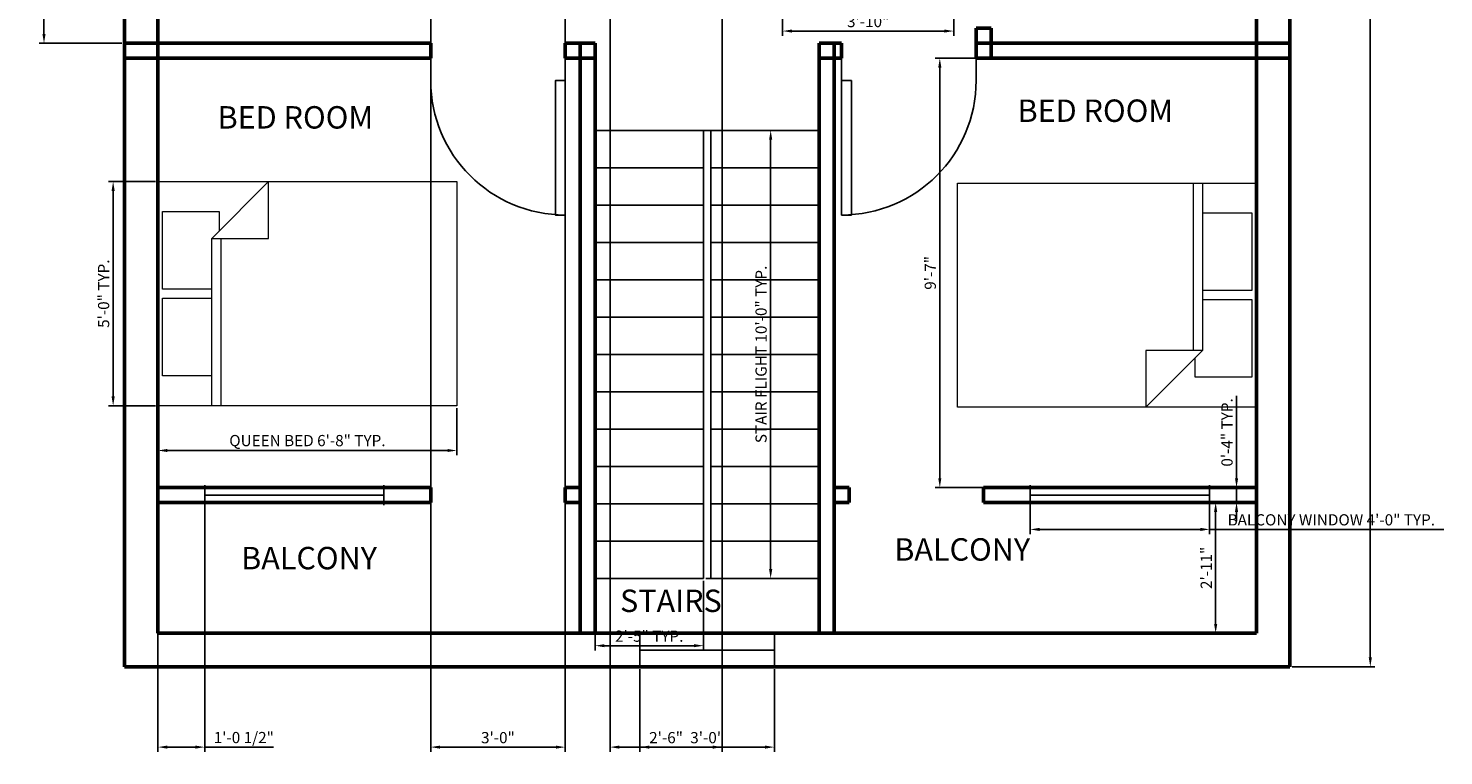
# Model space of a CAD drawing. Units: inches. Extents: x 1767 to 2185, y 3382 to 3854.
# Tile 1 of 4: x 1806 to 2185, y 3382 to 3577. Entities that reach past the tile are written whole.
import ezdxf

# ---------------------------------------------------------------- set-up
doc = ezdxf.new("R2010")
doc.units = ezdxf.units.IN
for name, color, linetype, lineweight in [('A-ANNO-DIMS', 2, 'Continuous', 18), ('A-AREA-IDEN', 7, 'Continuous', 25), ('A-DOOR', 3, 'Continuous', 25), ('A-FLOR-STRS', 7, 'Continuous', 25), ('A-FURN', 8, 'Continuous', 18), ('A-GLAZ', 4, 'Continuous', 25), ('A-WALL', 7, 'Continuous', 50)]:
    doc.layers.add(name, color=color, linetype=linetype, lineweight=lineweight)
doc.styles.get("Standard").update_dxf_attribs({"font": 'arial.ttf'})
doc.dimstyles.new('ISO-25', dxfattribs={"dimtxt": 3, "dimasz": 2.5, "dimexe": 1.25, "dimexo": 0.625, "dimtad": 1, "dimdec": 0, "dimlunit": 3, "dimtxsty": 'Standard', "dimcen": 2.5, "dimadec": 0, "dimazin": 0, "dimtfac": 1, "dimtdec": 0, "dimtmove": 0, "dimatfit": 3, "dimfxl": 1, "dimarcsym": 0})

# ---------------------------------------------------------------- blocks, each defined once
blk = doc.blocks.new('*U2')
for p, q in [((0, 0), (0, -100)), ((600, 0), (600, -100))]:
    blk.add_line(p, q)
blk.add_lwpolyline([(0, 0), (0, 600), (43.75, 600), (43.75, 0)], close=True)
blk.add_arc((0, 0), 600, 0, 90)
blk = doc.blocks.new('*U4')
for p, q in [((0, 100), (0, 0)), ((900, 100), (900, 0)), ((0, 50), (900, 50))]:
    blk.add_line(p, q)
blk = doc.blocks.new('Bed - Queen')
for p, q in [((0, -80.00003), (0, 0)), ((0, 0), (59.99999, 0)), ((59.99999, 0), (59.99999, -80.00003)), ((7.99999, -1.2), (28.79998, -1.2)), ((7.99999, -14.4), (7.99999, -1.2)), ((28.79998, -1.2), (28.79998, -14.4)), ((31.19999, -1.2), (51.99999, -1.2)), ((31.19999, -14.4), (31.19999, -1.2)), ((51.99999, -1.2), (51.99999, -16.4)), ((0, -14.4), (44.8, -14.4)), ((59.99999, -29.6), (44.8, -14.4)), ((44.8, -14.4), (44.8, -29.6)), ((44.8, -16.8), (0, -16.8)), ((51.99999, -16.4), (46.79936, -16.4)), ((44.8, -29.6), (59.99999, -29.6)), ((59.99999, -80.00003), (0, -80.00003))]:
    blk.add_line(p, q)
blk = doc.blocks.new('*D18')
at = {"layer": 'A-ANNO-DIMS', "color": 0, "lineweight": -2, "transparency": 16777216}
for p, q in [((2134.53, 3569.15), (2049.19, 3569.15)), ((2050.44, 3566.65), (2050.44, 3456.65)), ((2134.53, 3454.15), (2049.19, 3454.15))]:
    blk.add_line(p, q, dxfattribs=at)
at = {"layer": 'A-ANNO-DIMS', "color": 0, "transparency": 16777216}
for points in [[(2050.02, 3566.65), (2050.85, 3566.65), (2050.44, 3569.15)], [(2050.02, 3456.65), (2050.85, 3456.65), (2050.44, 3454.15)]]:
    blk.add_solid(points, dxfattribs=at)
at = {"layer": 'Defpoints', "color": 0, "transparency": 16777216}
for p in [(2135.16, 3569.15), (2050.44, 3454.15), (2135.16, 3454.15)]:
    blk.add_point(p, dxfattribs=at)
at = {"layer": 'A-ANNO-DIMS', "color": 0, "transparency": 16777216, "insert": (2048.28, 3511.65), "char_height": 3, "attachment_point": 5, "rotation": 90}
blk.add_mtext('9\'-7"', dxfattribs=at)
blk = doc.blocks.new('*D19')
at = {"layer": 'A-ANNO-DIMS', "color": 0, "lineweight": -2, "transparency": 16777216}
for p, q in [((2134.53, 3450.15), (2123.02, 3450.15)), ((2124.27, 3417.65), (2124.27, 3447.65)), ((2134.53, 3415.15), (2123.02, 3415.15))]:
    blk.add_line(p, q, dxfattribs=at)
at = {"layer": 'A-ANNO-DIMS', "color": 0, "transparency": 16777216}
for points in [[(2123.85, 3447.65), (2124.69, 3447.65), (2124.27, 3450.15)], [(2123.85, 3417.65), (2124.69, 3417.65), (2124.27, 3415.15)]]:
    blk.add_solid(points, dxfattribs=at)
at = {"layer": 'Defpoints', "color": 0, "transparency": 16777216}
for p in [(2124.27, 3450.15), (2135.16, 3450.15), (2135.16, 3415.15)]:
    blk.add_point(p, dxfattribs=at)
at = {"layer": 'A-ANNO-DIMS', "color": 0, "transparency": 16777216, "insert": (2122.14, 3432.65), "char_height": 3, "attachment_point": 5, "rotation": 90}
blk.add_mtext('2\'-11"', dxfattribs=at)
blk = doc.blocks.new('STAIR-FLIGHT-29IN-13-TREAD')
for p, q in [((0, 120), (29, 120)), ((29, 0), (29, 120)), ((0, 110), (29, 110)), ((0, 100), (29, 100)), ((0, 90), (29, 90)), ((0, 80), (29, 80)), ((0, 70), (29, 70)), ((0, 60), (29, 60)), ((0, 50), (29, 50)), ((0, 40), (29, 40)), ((0, 30), (29, 30)), ((0, 20), (29, 20)), ((0, 10), (29, 10)), ((0, 0), (29, 0))]:
    blk.add_line(p, q)
blk = doc.blocks.new('WIN-OPENING-48IN-WALL-4IN')
for p, q in [((48, 4), (0, 4)), ((0, 4), (0, 0)), ((48, 0), (48, 4))]:
    blk.add_line(p, q)
blk = doc.blocks.new('*D23')
at = {"layer": 'A-ANNO-DIMS', "color": 0, "lineweight": -2, "transparency": 16777216}
for p, q in [((1841.16, 3475.46), (1841.16, 3462.83)), ((1921.16, 3475.46), (1921.16, 3462.83)), ((1918.66, 3464.08), (1843.66, 3464.08))]:
    blk.add_line(p, q, dxfattribs=at)
at = {"layer": 'A-ANNO-DIMS', "color": 0, "transparency": 16777216}
for points in [[(1843.66, 3464.5), (1843.66, 3463.67), (1841.16, 3464.08)], [(1918.66, 3464.5), (1918.66, 3463.67), (1921.16, 3464.08)]]:
    blk.add_solid(points, dxfattribs=at)
at = {"layer": 'Defpoints', "color": 0, "transparency": 16777216}
for p in [(1841.16, 3476.08), (1921.16, 3476.08), (1841.16, 3464.08)]:
    blk.add_point(p, dxfattribs=at)
at = {"layer": 'A-ANNO-DIMS', "color": 0, "transparency": 16777216, "insert": (1881.16, 3466.35), "char_height": 3, "attachment_point": 5}
blk.add_mtext('QUEEN BED 6\'-8" TYP.', dxfattribs=at)
blk = doc.blocks.new('*D24')
at = {"layer": 'A-ANNO-DIMS', "color": 0, "lineweight": -2, "transparency": 16777216}
for p, q in [((1840.53, 3536.08), (1827.91, 3536.08)), ((1829.16, 3478.58), (1829.16, 3533.58)), ((1840.53, 3476.08), (1827.91, 3476.08))]:
    blk.add_line(p, q, dxfattribs=at)
at = {"layer": 'A-ANNO-DIMS', "color": 0, "transparency": 16777216}
for points in [[(1828.74, 3533.58), (1829.58, 3533.58), (1829.16, 3536.08)], [(1828.74, 3478.58), (1829.58, 3478.58), (1829.16, 3476.08)]]:
    blk.add_solid(points, dxfattribs=at)
at = {"layer": 'Defpoints', "color": 0, "transparency": 16777216}
for p in [(1829.16, 3536.08), (1841.16, 3536.08), (1841.16, 3476.08)]:
    blk.add_point(p, dxfattribs=at)
at = {"layer": 'A-ANNO-DIMS', "color": 0, "transparency": 16777216, "insert": (1827, 3506.08), "char_height": 3, "attachment_point": 5, "rotation": 90}
blk.add_mtext('5\'-0" TYP.', dxfattribs=at)
blk = doc.blocks.new('*D25')
at = {"layer": 'A-ANNO-DIMS', "color": 0, "lineweight": -2, "transparency": 16777216}
for p, q in [((1987.78, 3549.81), (2006.41, 3549.81)), ((2005.16, 3432.31), (2005.16, 3547.31)), ((1987.78, 3429.81), (2006.41, 3429.81))]:
    blk.add_line(p, q, dxfattribs=at)
at = {"layer": 'A-ANNO-DIMS', "color": 0, "transparency": 16777216}
for points in [[(2004.74, 3547.31), (2005.58, 3547.31), (2005.16, 3549.81)], [(2004.74, 3432.31), (2005.58, 3432.31), (2005.16, 3429.81)]]:
    blk.add_solid(points, dxfattribs=at)
at = {"layer": 'Defpoints', "color": 0, "transparency": 16777216}
for p in [(1987.16, 3549.81), (2005.16, 3549.81), (1987.16, 3429.81)]:
    blk.add_point(p, dxfattribs=at)
at = {"layer": 'A-ANNO-DIMS', "color": 0, "transparency": 16777216, "insert": (2002.98, 3489.81), "char_height": 3, "attachment_point": 5, "rotation": 90}
blk.add_mtext('STAIR FLIGHT 10\'-0" TYP.', dxfattribs=at)
blk = doc.blocks.new('*D26')
at = {"layer": 'A-ANNO-DIMS', "color": 0, "lineweight": -2, "transparency": 16777216}
for p, q in [((1958.16, 3429.19), (1958.16, 3410.56)), ((1987.16, 3429.19), (1987.16, 3410.56)), ((1960.66, 3411.81), (1984.66, 3411.81))]:
    blk.add_line(p, q, dxfattribs=at)
at = {"layer": 'A-ANNO-DIMS', "color": 0, "transparency": 16777216}
for points in [[(1960.66, 3412.23), (1960.66, 3411.4), (1958.16, 3411.81)], [(1984.66, 3412.23), (1984.66, 3411.4), (1987.16, 3411.81)]]:
    blk.add_solid(points, dxfattribs=at)
at = {"layer": 'Defpoints', "color": 0, "transparency": 16777216}
for p in [(1958.16, 3429.81), (1987.16, 3429.81), (1987.16, 3411.81)]:
    blk.add_point(p, dxfattribs=at)
at = {"layer": 'A-ANNO-DIMS', "color": 0, "transparency": 16777216, "insert": (1972.66, 3413.97), "char_height": 3, "attachment_point": 5}
blk.add_mtext('2\'-5" TYP.', dxfattribs=at)
blk = doc.blocks.new('*D29')
at = {"layer": 'A-ANNO-DIMS', "color": 0, "lineweight": -2, "transparency": 16777216}
for p, q in [((2074.66, 3449.53), (2074.66, 3441.7)), ((2122.66, 3449.53), (2122.66, 3441.7)), ((2077.16, 3442.95), (2120.16, 3442.95)), ((2122.66, 3442.95), (2185.31, 3442.95))]:
    blk.add_line(p, q, dxfattribs=at)
at = {"layer": 'A-ANNO-DIMS', "color": 0, "transparency": 16777216}
for points in [[(2077.16, 3443.37), (2077.16, 3442.53), (2074.66, 3442.95)], [(2120.16, 3443.37), (2120.16, 3442.53), (2122.66, 3442.95)]]:
    blk.add_solid(points, dxfattribs=at)
at = {"layer": 'Defpoints', "color": 0, "transparency": 16777216}
for p in [(2074.66, 3450.15), (2122.66, 3450.15), (2122.66, 3442.95)]:
    blk.add_point(p, dxfattribs=at)
at = {"layer": 'A-ANNO-DIMS', "color": 0, "transparency": 16777216, "insert": (2155.23, 3445.13), "char_height": 3, "attachment_point": 5}
blk.add_mtext('BALCONY WINDOW 4\'-0" TYP.', dxfattribs=at)
blk = doc.blocks.new('*D30')
at = {"layer": 'A-ANNO-DIMS', "color": 0, "lineweight": -2, "transparency": 16777216}
for p, q in [((2129.86, 3456.65), (2129.86, 3478.69)), ((2123.28, 3454.15), (2131.11, 3454.15)), ((2129.86, 3450.15), (2129.86, 3454.15)), ((2123.28, 3450.15), (2131.11, 3450.15)), ((2129.86, 3447.65), (2129.86, 3445.15))]:
    blk.add_line(p, q, dxfattribs=at)
at = {"layer": 'A-ANNO-DIMS', "color": 0, "transparency": 16777216}
for points in [[(2129.44, 3456.65), (2130.28, 3456.65), (2129.86, 3454.15)], [(2129.44, 3447.65), (2130.28, 3447.65), (2129.86, 3450.15)]]:
    blk.add_solid(points, dxfattribs=at)
at = {"layer": 'Defpoints', "color": 0, "transparency": 16777216}
for p in [(2122.66, 3454.15), (2129.86, 3454.15), (2122.66, 3450.15)]:
    blk.add_point(p, dxfattribs=at)
at = {"layer": 'A-ANNO-DIMS', "color": 0, "transparency": 16777216, "insert": (2127.7, 3468.92), "char_height": 3, "attachment_point": 5, "rotation": 90}
blk.add_mtext('0\'-4" TYP.', dxfattribs=at)
blk = doc.blocks.new('*D32')
at = {"layer": 'A-ANNO-DIMS', "color": 0, "lineweight": -2, "transparency": 16777216}
for p, q in [((2008.34, 3587.16), (2008.34, 3575.16)), ((2054.18, 3587.16), (2054.18, 3575.16)), ((2051.68, 3576.41), (2010.84, 3576.41))]:
    blk.add_line(p, q, dxfattribs=at)
at = {"layer": 'A-ANNO-DIMS', "color": 0, "transparency": 16777216}
for points in [[(2010.84, 3576.83), (2010.84, 3576), (2008.34, 3576.41)], [(2051.68, 3576.83), (2051.68, 3576), (2054.18, 3576.41)]]:
    blk.add_solid(points, dxfattribs=at)
at = {"layer": 'Defpoints', "color": 0, "transparency": 16777216}
for p in [(2008.34, 3587.79), (2054.18, 3587.79), (2008.34, 3576.41)]:
    blk.add_point(p, dxfattribs=at)
at = {"layer": 'A-ANNO-DIMS', "color": 0, "transparency": 16777216, "insert": (2031.26, 3578.57), "char_height": 3, "attachment_point": 5}
blk.add_mtext('3\'-10"', dxfattribs=at)
blk = doc.blocks.new('*D40')
at = {"layer": 'A-ANNO-DIMS', "color": 0, "lineweight": -2, "transparency": 16777216}
for p, q in [((2144.78, 3826.15), (2166.91, 3826.15)), ((2165.66, 3408.65), (2165.66, 3823.65)), ((2144.78, 3406.15), (2166.91, 3406.15))]:
    blk.add_line(p, q, dxfattribs=at)
at = {"layer": 'A-ANNO-DIMS', "color": 0, "transparency": 16777216}
for points in [[(2165.25, 3823.65), (2166.08, 3823.65), (2165.66, 3826.15)], [(2165.25, 3408.65), (2166.08, 3408.65), (2165.66, 3406.15)]]:
    blk.add_solid(points, dxfattribs=at)
at = {"layer": 'Defpoints', "color": 0, "transparency": 16777216}
for p in [(2144.16, 3826.15), (2165.66, 3826.15), (2144.16, 3406.15)]:
    blk.add_point(p, dxfattribs=at)
at = {"layer": 'A-ANNO-DIMS', "color": 0, "transparency": 16777216, "insert": (2163.51, 3616.15), "char_height": 3, "attachment_point": 5, "rotation": 90}
blk.add_mtext('35\'-0"', dxfattribs=at)
blk = doc.blocks.new('*D41')
at = {"layer": 'A-ANNO-DIMS', "color": 0, "lineweight": -2, "transparency": 16777216}
for p, q in [((1840.53, 3669.15), (1809.4, 3669.15)), ((1810.65, 3575.65), (1810.65, 3666.65)), ((1831.53, 3573.15), (1809.4, 3573.15))]:
    blk.add_line(p, q, dxfattribs=at)
at = {"layer": 'A-ANNO-DIMS', "color": 0, "transparency": 16777216}
for points in [[(1810.24, 3666.65), (1811.07, 3666.65), (1810.65, 3669.15)], [(1810.24, 3575.65), (1811.07, 3575.65), (1810.65, 3573.15)]]:
    blk.add_solid(points, dxfattribs=at)
at = {"layer": 'Defpoints', "color": 0, "transparency": 16777216}
for p in [(1810.65, 3669.15), (1841.16, 3669.15), (1832.16, 3573.15)]:
    blk.add_point(p, dxfattribs=at)
at = {"layer": 'A-ANNO-DIMS', "color": 0, "transparency": 16777216, "insert": (1808.5, 3621.15), "char_height": 3, "attachment_point": 5, "rotation": 90}
blk.add_mtext('8\'-0"', dxfattribs=at)
blk = doc.blocks.new('*D42')
at = {"layer": 'A-ANNO-DIMS', "color": 0, "lineweight": -2, "transparency": 16777216}
for p, q in [((1914.16, 3668.53), (1914.16, 3383.4)), ((1950.16, 3668.53), (1950.16, 3383.4)), ((1916.66, 3384.65), (1947.66, 3384.65))]:
    blk.add_line(p, q, dxfattribs=at)
at = {"layer": 'A-ANNO-DIMS', "color": 0, "transparency": 16777216}
for points in [[(1916.66, 3385.06), (1916.66, 3384.23), (1914.16, 3384.65)], [(1947.66, 3385.06), (1947.66, 3384.23), (1950.16, 3384.65)]]:
    blk.add_solid(points, dxfattribs=at)
at = {"layer": 'Defpoints', "color": 0, "transparency": 16777216}
for p in [(1914.16, 3669.15), (1950.16, 3669.15), (1950.16, 3384.65)]:
    blk.add_point(p, dxfattribs=at)
at = {"layer": 'A-ANNO-DIMS', "color": 0, "transparency": 16777216, "insert": (1932.16, 3386.8), "char_height": 3, "attachment_point": 5}
blk.add_mtext('3\'-0"', dxfattribs=at)
blk = doc.blocks.new('*D43')
at = {"layer": 'A-ANNO-DIMS', "color": 0, "lineweight": -2, "transparency": 16777216}
for p, q in [((1962.16, 3668.53), (1962.16, 3383.4)), ((1992.16, 3668.53), (1992.16, 3383.4)), ((1964.66, 3384.65), (1989.66, 3384.65))]:
    blk.add_line(p, q, dxfattribs=at)
at = {"layer": 'A-ANNO-DIMS', "color": 0, "transparency": 16777216}
for points in [[(1964.66, 3385.06), (1964.66, 3384.23), (1962.16, 3384.65)], [(1989.66, 3385.06), (1989.66, 3384.23), (1992.16, 3384.65)]]:
    blk.add_solid(points, dxfattribs=at)
at = {"layer": 'Defpoints', "color": 0, "transparency": 16777216}
for p in [(1962.16, 3669.15), (1992.16, 3669.15), (1992.16, 3384.65)]:
    blk.add_point(p, dxfattribs=at)
at = {"layer": 'A-ANNO-DIMS', "color": 0, "transparency": 16777216, "insert": (1977.16, 3386.8), "char_height": 3, "attachment_point": 5}
blk.add_mtext('2\'-6"', dxfattribs=at)
blk = doc.blocks.new('*D47')
at = {"layer": 'A-ANNO-DIMS', "color": 0, "lineweight": -2, "transparency": 16777216}
for p, q in [((1970.16, 3405.53), (1970.16, 3383.4)), ((2006.16, 3405.53), (2006.16, 3383.4)), ((1972.66, 3384.65), (2003.66, 3384.65))]:
    blk.add_line(p, q, dxfattribs=at)
at = {"layer": 'A-ANNO-DIMS', "color": 0, "transparency": 16777216}
for points in [[(1972.66, 3385.06), (1972.66, 3384.23), (1970.16, 3384.65)], [(2003.66, 3385.06), (2003.66, 3384.23), (2006.16, 3384.65)]]:
    blk.add_solid(points, dxfattribs=at)
at = {"layer": 'Defpoints', "color": 0, "transparency": 16777216}
for p in [(1970.16, 3406.15), (2006.16, 3406.15), (2006.16, 3384.65)]:
    blk.add_point(p, dxfattribs=at)
at = {"layer": 'A-ANNO-DIMS', "color": 0, "transparency": 16777216, "insert": (1988.16, 3386.8), "char_height": 3, "attachment_point": 5}
blk.add_mtext('3\'-0"', dxfattribs=at)
blk = doc.blocks.new('*D49')
at = {"layer": 'A-ANNO-DIMS', "color": 0, "lineweight": -2, "transparency": 16777216}
for p, q in [((1841.16, 3449.53), (1841.16, 3383.4)), ((1853.66, 3449.53), (1853.66, 3383.4)), ((1843.66, 3384.65), (1851.16, 3384.65)), ((1853.66, 3384.65), (1872.09, 3384.65))]:
    blk.add_line(p, q, dxfattribs=at)
at = {"layer": 'A-ANNO-DIMS', "color": 0, "transparency": 16777216}
for points in [[(1843.66, 3385.06), (1843.66, 3384.23), (1841.16, 3384.65)], [(1851.16, 3385.06), (1851.16, 3384.23), (1853.66, 3384.65)]]:
    blk.add_solid(points, dxfattribs=at)
at = {"layer": 'Defpoints', "color": 0, "transparency": 16777216}
for p in [(1841.16, 3450.15), (1853.66, 3450.15), (1853.66, 3384.65)]:
    blk.add_point(p, dxfattribs=at)
at = {"layer": 'A-ANNO-DIMS', "color": 0, "transparency": 16777216, "insert": (1864.13, 3386.82), "char_height": 3, "attachment_point": 5}
blk.add_mtext('1\'-0 1/2"', dxfattribs=at)

msp = doc.modelspace()

# ---------------------------------------------------------------- linework, layer by layer
at = {"layer": 'A-FLOR-STRS'}
msp.add_line((1987.16, 3549.81), (1989.16, 3549.81), dxfattribs=at)
at = {"layer": 'A-GLAZ'}
for p, q in [((1970.16, 3415.15), (1970.16, 3406.15)), ((2006.16, 3406.15), (2006.16, 3415.15)), ((1970.16, 3406.15), (2006.16, 3406.15))]:
    msp.add_line(p, q, dxfattribs=at)
at = {"layer": 'A-WALL'}
for p, q in [((1832.16, 3406.15), (1832.16, 3826.15)), ((2144.16, 3826.15), (2144.16, 3406.15)), ((1841.16, 3415.15), (1841.16, 3817.15)), ((2135.16, 3817.15), (2135.16, 3415.15)), ((2060.16, 3577.15), (2064.16, 3577.15)), ((2060.16, 3577.15), (2060.16, 3569.15)), ((2064.16, 3577.15), (2064.16, 3569.15)), ((1832.16, 3573.15), (1914.16, 3573.15)), ((1914.16, 3573.15), (1914.16, 3569.15)), ((1950.16, 3569.15), (1950.16, 3573.15)), ((1950.16, 3573.15), (1958.16, 3573.15)), ((1954.16, 3415.15), (1954.16, 3573.15)), ((1958.16, 3415.15), (1958.16, 3573.15)), ((2018.16, 3573.15), (2018.16, 3415.15)), ((2018.16, 3573.15), (2024.16, 3573.15)), ((2022.16, 3573.15), (2022.16, 3415.15)), ((2024.16, 3569.15), (2024.16, 3573.15)), ((2060.16, 3573.15), (2060.16, 3569.15)), ((2060.16, 3573.15), (2144.16, 3573.15)), ((1832.16, 3569.15), (1914.16, 3569.15)), ((1950.16, 3569.15), (1958.16, 3569.15)), ((2018.16, 3569.15), (2024.16, 3569.15)), ((2060.16, 3569.15), (2144.16, 3569.15)), ((1914.16, 3454.15), (1841.16, 3454.15)), ((1914.16, 3454.15), (1914.16, 3450.15)), ((1954.16, 3454.15), (1950.16, 3454.15)), ((1950.16, 3450.15), (1950.16, 3454.15)), ((2026.16, 3454.15), (2022.16, 3454.15)), ((2026.16, 3454.15), (2026.16, 3450.15)), ((2135.16, 3454.15), (2062.16, 3454.15)), ((2062.16, 3450.15), (2062.16, 3454.15)), ((1914.16, 3450.15), (1841.16, 3450.15)), ((1954.16, 3450.15), (1950.16, 3450.15)), ((2026.16, 3450.15), (2022.16, 3450.15)), ((2135.16, 3450.15), (2062.16, 3450.15)), ((2135.16, 3415.15), (1841.16, 3415.15)), ((2144.16, 3406.15), (1832.16, 3406.15))]:
    msp.add_line(p, q, dxfattribs=at)

# ---------------------------------------------------------------- block references
at = {"layer": 'A-DOOR', "yscale": 0.0599999999999998, "zscale": 0.0599999999999998, "rotation": 180}
for p, xscale in [((1950.16, 3563.15), 0.0599999999999998), ((2024.16, 3563.15), -0.0599999999999998)]:
    msp.add_blockref('*U2', p, dxfattribs=dict(at, xscale=xscale))
at = {"layer": 'A-FLOR-STRS'}
msp.add_blockref('STAIR-FLIGHT-29IN-13-TREAD', (1958.16, 3429.81), dxfattribs=at)
at = {"layer": 'A-FLOR-STRS', "rotation": 180}
msp.add_blockref('STAIR-FLIGHT-29IN-13-TREAD', (2018.16, 3549.81), dxfattribs=at)
at = {"layer": 'A-FURN'}
for p, rotation in [((1841.16, 3476.08), 90), ((2135.16, 3535.7), 269.9999999999998)]:
    msp.add_blockref('Bed - Queen', p, dxfattribs=dict(at, rotation=rotation))
at = {"layer": 'A-GLAZ', "xscale": 0.0533333333333335, "yscale": 0.0533333333333335, "zscale": 0.0533333333333335}
for p in [(1853.66, 3449.48), (2074.66, 3449.48)]:
    msp.add_blockref('*U4', p, dxfattribs=at)
at = {"layer": 'A-GLAZ'}
for p in [(1853.66, 3450.15), (2074.66, 3450.15)]:
    msp.add_blockref('WIN-OPENING-48IN-WALL-4IN', p, dxfattribs=at)
at = {"layer": 'A-GLAZ', "xscale": 0.0399999999999999, "yscale": 0.0399999999999999, "zscale": 0.0399999999999999, "rotation": 180}
msp.add_blockref('*U4', (2006.16, 3412.65), dxfattribs=at)

# ---------------------------------------------------------------- texts
at = {"layer": 'A-AREA-IDEN'}
for s, p in [('BED ROOM', (2071.25, 3552.08)), ('BED ROOM', (1857.12, 3550.3)), ('BALCONY', (2038.25, 3434.59)), ('BALCONY', (1863.42, 3432.27)), ('STAIRS', (1964.84, 3420.83))]:
    msp.add_text(s, height=6, dxfattribs=at).set_placement(p)

# ---------------------------------------------------------------- dimensions: what is measured, and where the dimension line sits
at = {"layer": 'A-ANNO-DIMS'}
for base, p1, p2, angle, override, picture, middle in [((2165.66, 3826.15), (2144.16, 3406.15), (2144.16, 3826.15), 90, {"dimdec": 1, "dimlfac": 1, "dimrnd": 0, "dimzin": 1, "dimdsep": 46, "dimlunit": 4, "dimfrac": 2}, '*D40', (2163.51, 3616.15)), ((1810.65, 3669.15), (1832.16, 3573.15), (1841.16, 3669.15), 90, {"dimdec": 1, "dimlfac": 1, "dimrnd": 0, "dimzin": 1, "dimdsep": 46, "dimlunit": 4, "dimfrac": 2}, '*D41', (1808.5, 3621.15)), ((2008.34, 3576.41), (2054.18, 3587.79), (2008.34, 3587.79), 180, {"dimdec": 1, "dimlfac": 1, "dimrnd": 0, "dimzin": 1, "dimdsep": 46, "dimlunit": 4, "dimfrac": 2}, '*D32', (2031.26, 3578.57)), ((2050.44, 3454.15), (2135.16, 3569.15), (2135.16, 3454.15), 90, {"dimclrd": 0, "dimclre": 0, "dimclrt": 0}, '*D18', (2048.28, 3511.65)), ((2124.27, 3450.15), (2135.16, 3415.15), (2135.16, 3450.15), 90, {"dimclrd": 0, "dimclre": 0, "dimclrt": 0}, '*D19', (2122.14, 3432.65))]:
    dim = msp.add_linear_dim(base=base, p1=p1, p2=p2, angle=angle, dimstyle='ISO-25', override=override, dxfattribs=at)
    dim.commit()
    dim.dimension.update_dxf_attribs({"geometry": picture, "text_midpoint": middle})
for base, p1, p2, picture, middle in [((1950.16, 3384.65), (1914.16, 3669.15), (1950.16, 3669.15), '*D42', (1932.16, 3386.8)), ((1992.16, 3384.65), (1962.16, 3669.15), (1992.16, 3669.15), '*D43', (1977.16, 3386.8)), ((1853.66, 3384.65), (1841.16, 3450.15), (1853.66, 3450.15), '*D49', (1864.13, 3386.82)), ((2006.16, 3384.65), (1970.16, 3406.15), (2006.16, 3406.15), '*D47', (1988.16, 3386.8))]:
    dim = msp.add_linear_dim(base=base, p1=p1, p2=p2, dimstyle='ISO-25', override={"dimdec": 1, "dimlfac": 1, "dimrnd": 0, "dimzin": 1, "dimdsep": 46, "dimlunit": 4, "dimfrac": 2}, dxfattribs=at)
    dim.commit()
    dim.dimension.update_dxf_attribs({"geometry": picture, "text_midpoint": middle})
for base, p1, p2, angle, text, picture, middle in [((2005.16, 3549.81), (1987.16, 3429.81), (1987.16, 3549.81), 90, 'STAIR FLIGHT <> TYP.', '*D25', (2002.98, 3489.81)), ((1829.16, 3536.08), (1841.16, 3476.08), (1841.16, 3536.08), 90, '<> TYP.', '*D24', (1827, 3506.08)), ((2129.86, 3454.15), (2122.66, 3450.15), (2122.66, 3454.15), 90, '<> TYP.', '*D30', (2127.7, 3468.92)), ((1841.16, 3464.08), (1921.16, 3476.08), (1841.16, 3476.08), 180, 'QUEEN BED <> TYP.', '*D23', (1881.16, 3466.35))]:
    dim = msp.add_linear_dim(base=base, p1=p1, p2=p2, angle=angle, text=text, dimstyle='ISO-25', override={"dimdec": 1, "dimlfac": 1, "dimrnd": 0, "dimzin": 1, "dimdsep": 46, "dimlunit": 4, "dimfrac": 2}, dxfattribs=at)
    dim.commit()
    dim.dimension.update_dxf_attribs({"geometry": picture, "text_midpoint": middle})
for base, p1, p2, text, picture, middle in [((2122.66, 3442.95), (2074.66, 3450.15), (2122.66, 3450.15), 'BALCONY WINDOW <> TYP.', '*D29', (2155.23, 3445.13)), ((1987.16, 3411.81), (1958.16, 3429.81), (1987.16, 3429.81), '<> TYP.', '*D26', (1972.66, 3413.97))]:
    dim = msp.add_linear_dim(base=base, p1=p1, p2=p2, text=text, dimstyle='ISO-25', override={"dimdec": 1, "dimlfac": 1, "dimrnd": 0, "dimzin": 1, "dimdsep": 46, "dimlunit": 4, "dimfrac": 2}, dxfattribs=at)
    dim.commit()
    dim.dimension.update_dxf_attribs({"geometry": picture, "text_midpoint": middle})

doc.saveas('drawing.dxf')
